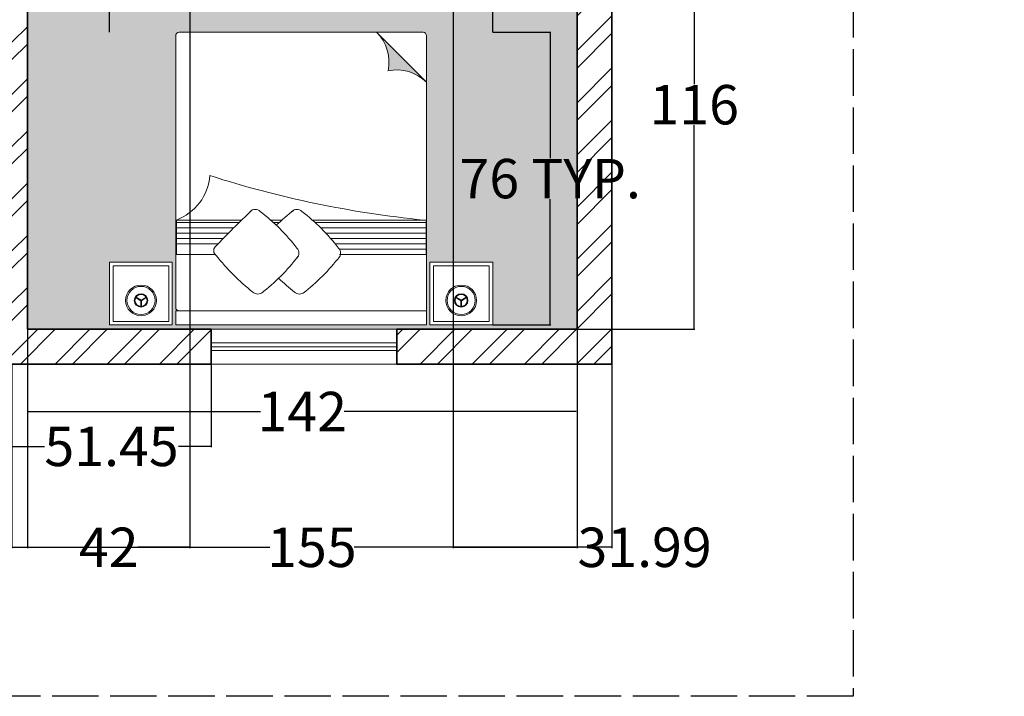
# Model space of a CAD drawing. Units: inches. Extents: x 1410 to 1959, y 5441 to 5968.
# Tile 3 of 5: x 1705 to 1959, y 5441 to 5615. Entities that reach past the tile are written whole.
import ezdxf

# ---------------------------------------------------------------- set-up
doc = ezdxf.new("R2010")
doc.units = ezdxf.units.IN
doc.linetypes.add('ACAD_ISO02W100', pattern=[15, 12, -3])
doc.layers.get('Defpoints').update_dxf_attribs({"linetype": 'ACAD_ISO02W100'})
for name, color, linetype, lineweight in [('00 FURNITURE', 15, 'Continuous', 15), ('A-ANNO-DIMS', 2, 'Continuous', 18), ('A-WALL', 7, 'Continuous', 35), ('A-WALL-PATT', 8, 'Continuous', 13), ('WINDOW', 160, 'Continuous', 13)]:
    doc.layers.add(name, color=color, linetype=linetype, lineweight=lineweight)
doc.layers.add('A-FLOR-PATT', color=9, linetype='Continuous', lineweight=9, true_color=0xafd9aa)
doc.styles.get("Standard").update_dxf_attribs({"font": 'arial.ttf'})
doc.dimstyles.get("Standard").update_dxf_attribs({"dimtxt": 10.18, "dimasz": 0.18, "dimexe": 0.18, "dimexo": 0.0625, "dimgap": 0.09, "dimtad": 0, "dimtih": 1, "dimtoh": 1, "dimdec": 0, "dimzin": 0, "dimdsep": 46, "dimlunit": 3, "dimtxsty": 'Standard', "dimcen": 0.09, "dimadec": 0, "dimazin": 0, "dimtfac": 1, "dimtdec": 0, "dimtofl": 0, "dimtmove": 0, "dimatfit": 3, "dimfxl": 1, "dimtolj": 1, "dimtzin": 0, "dimarcsym": 0})

# ---------------------------------------------------------------- blocks, each defined once
blk = doc.blocks.new('RGWTG')
at = {"layer": '00 FURNITURE'}
for p, q in [((578.23, 3473.51), (577.36, 3475.01)), ((578.36, 3473.58), (577.49, 3475.09)), ((578.23, 3473.58), (577.36, 3472.08)), ((578.36, 3473.51), (577.49, 3472)), ((578.29, 3473.62), (580.03, 3473.62)), ((578.29, 3473.47), (580.03, 3473.47)), ((521.93, 3464.58), (509.03, 3451.68)), ((509.03, 3422.63), (509.03, 3463.68)), ((509.93, 3464.58), (566.4, 3464.58)), ((557.53, 3463.84), (557.53, 3464.49)), ((557.53, 3464.49), (566.4, 3464.49)), ((558.2, 3464.49), (558.2, 3435.82)), ((559.57, 3464.49), (559.57, 3437.25)), ((560.94, 3464.49), (560.94, 3438.58)), ((562.3, 3464.49), (562.3, 3439.83)), ((563.67, 3464.49), (563.67, 3440.99)), ((565.04, 3464.49), (565.04, 3442.08)), ((566.4, 3464.58), (580.98, 3464.58)), ((566.4, 3464.49), (566.4, 3442.08)), ((566.4, 3464.49), (566.4, 3463.84)), ((580.98, 3464.58), (580.98, 3416.72)), ((558.2, 3426.48), (558.2, 3425.04)), ((509.03, 3400.68), (509.03, 3422.63)), ((580.98, 3416.72), (580.98, 3400.68)), ((558.2, 3416.13), (558.2, 3399.95)), ((559.57, 3414.75), (559.57, 3399.95)), ((560.94, 3413.39), (560.94, 3399.95)), ((562.3, 3412.04), (562.3, 3399.95)), ((563.67, 3410.72), (563.67, 3399.95)), ((580.08, 3399.78), (509.93, 3399.78)), ((557.53, 3399.95), (557.53, 3400.6)), ((566.4, 3399.95), (557.53, 3399.95)), ((566.4, 3400.6), (566.4, 3399.95)), ((578.23, 3390.78), (577.36, 3392.29)), ((578.36, 3390.86), (577.49, 3392.36)), ((578.23, 3390.86), (577.36, 3389.36)), ((578.36, 3390.78), (577.49, 3389.28)), ((578.29, 3390.9), (580.03, 3390.9)), ((578.29, 3390.74), (580.03, 3390.74))]:
    blk.add_line(p, q, dxfattribs=at)
for points in [[(568.43, 3465.48), (584.63, 3465.48), (584.63, 3481.68), (568.43, 3481.68)], [(569.33, 3466.38), (583.73, 3466.38), (583.73, 3480.78), (569.33, 3480.78)], [(580.98, 3399.78), (584.63, 3399.78), (584.63, 3464.58), (580.98, 3464.58)], [(568.43, 3398.88), (584.63, 3398.88), (584.63, 3382.68), (568.43, 3382.68)], [(569.33, 3397.98), (583.73, 3397.98), (583.73, 3383.58), (569.33, 3383.58)]]:
    blk.add_lwpolyline(points, close=True, dxfattribs=at)
for points in [[(566.52, 3464.49), (557.53, 3464.49), (557.53, 3435.08)], [(557.53, 3427.21), (557.53, 3424.3)], [(557.53, 3416.82), (557.53, 3399.95), (566.4, 3399.95), (566.4, 3409.94)]]:
    blk.add_lwpolyline(points, dxfattribs=at)
for centre, radius in [((578.29, 3473.54), 3.97), ((578.29, 3473.54), 3.63), ((578.29, 3473.54), 1.74), ((578.29, 3473.54), 1.56), ((578.29, 3390.82), 3.97), ((578.29, 3390.82), 3.63), ((578.29, 3390.82), 1.74), ((578.29, 3390.82), 1.56)]:
    blk.add_circle(centre, radius, dxfattribs=at)
for centre, radius, start, end in [((509.93, 3463.68), 0.9, 90, 180), ((529.65, 3456.88), 10.9, 135.0361, 191.9278), ((290.56, 3490.52), 268.3, 342.2214, 354.2925), ((516.73, 3443.97), 10.9, 78.0722, 134.9639), ((566.05, 3440.57), 1.82, 45, 135), ((533.58, 3399.31), 54.32, 37.931, 52.069), ((598.15, 3399.01), 54.32, 127.931, 142.069), ((556.59, 3431.11), 1.82, 135, 225), ((574.84, 3431.77), 1.82, 315, 45), ((597.87, 3463.6), 54.32, 217.931, 224.141), ((598.15, 3388.23), 54.32, 127.931, 142.069), ((566.05, 3429.78), 1.82, 45, 135), ((533.58, 3388.53), 54.32, 37.931, 52.069), ((533.28, 3463.88), 54.32, 316.32, 322.069), ((556.59, 3420.33), 1.82, 135, 225), ((574.84, 3420.99), 1.82, 315, 45), ((765.33, 3619.75), 290.45, 223.6069, 226.2326), ((533.28, 3453.1), 54.32, 307.931, 322.069), ((565.44, 3411.05), 1.47, 225.9674, 326.8337), ((545.02, 3395.29), 13.35, 20.4224, 85.5825), ((509.93, 3400.68), 0.9, 180, 270), ((580.08, 3400.68), 0.9, 270, 0)]:
    blk.add_arc(centre, radius, start, end, dxfattribs=at)
blk = doc.blocks.new('WIN-48IN')
for p, q in [((48, 9), (0, 9)), ((0, 5.5), (48, 5.5)), ((0, 4.5), (48, 4.5)), ((0, 3.5), (48, 3.5)), ((0, 0), (48, 0))]:
    blk.add_line(p, q)
blk = doc.blocks.new('*D14')
at = {"layer": 'A-ANNO-DIMS', "color": 0, "lineweight": -2, "transparency": 16777216}
for p, q in [((1728.31, 5612.14), (1728.31, 5627.11)), ((1728.49, 5626.93), (1827.13, 5626.93)), ((1827.31, 5612.14), (1827.31, 5627.11)), ((1827.31, 5626.93), (1827.49, 5626.93))]:
    blk.add_line(p, q, dxfattribs=at)
at = {"layer": 'A-ANNO-DIMS', "color": 0, "transparency": 16777216}
for points in [[(1728.49, 5626.96), (1728.49, 5626.9), (1728.31, 5626.93)], [(1827.13, 5626.96), (1827.13, 5626.9), (1827.31, 5626.93)]]:
    blk.add_solid(points, dxfattribs=at)
at = {"layer": 'Defpoints', "color": 0, "transparency": 16777216}
for p in [(1827.31, 5626.93), (1728.31, 5612.08), (1827.31, 5612.08)]:
    blk.add_point(p, dxfattribs=at)
at = {"layer": 'A-ANNO-DIMS', "color": 0, "transparency": 16777216, "insert": (1896.77, 5626.93), "char_height": 10.18, "attachment_point": 5}
blk.add_mtext('\\A1;BED GROUP 99 TYP.', dxfattribs=at)
blk = doc.blocks.new('*D15')
at = {"layer": 'A-ANNO-DIMS', "color": 0, "lineweight": -2, "transparency": 16777216}
for p, q in [((1827.37, 5612.08), (1842.34, 5612.08)), ((1842.16, 5611.9), (1842.16, 5579.57)), ((1842.16, 5536.66), (1842.16, 5568.99)), ((1827.37, 5536.48), (1842.34, 5536.48))]:
    blk.add_line(p, q, dxfattribs=at)
at = {"layer": 'A-ANNO-DIMS', "color": 0, "transparency": 16777216}
for points in [[(1842.13, 5611.9), (1842.19, 5611.9), (1842.16, 5612.08)], [(1842.13, 5536.66), (1842.19, 5536.66), (1842.16, 5536.48)]]:
    blk.add_solid(points, dxfattribs=at)
at = {"layer": 'Defpoints', "color": 0, "transparency": 16777216}
for p in [(1827.31, 5612.08), (1827.31, 5536.48), (1842.16, 5536.48)]:
    blk.add_point(p, dxfattribs=at)
at = {"layer": 'A-ANNO-DIMS', "color": 0, "transparency": 16777216, "insert": (1842.16, 5574.28), "char_height": 10.18, "attachment_point": 5}
blk.add_mtext('\\A1;76 TYP.', dxfattribs=at)
blk = doc.blocks.new('*D26')
at = {"layer": 'A-ANNO-DIMS', "color": 0, "lineweight": -2, "transparency": 16777216}
for p, q in [((1703.09, 5526.3), (1703.09, 5478.87)), ((1858.09, 5526.3), (1858.09, 5478.87)), ((1703.27, 5479.05), (1769.7, 5479.05)), ((1857.91, 5479.05), (1791.49, 5479.05))]:
    blk.add_line(p, q, dxfattribs=at)
at = {"layer": 'A-ANNO-DIMS', "color": 0, "transparency": 16777216}
for points in [[(1703.27, 5479.08), (1703.27, 5479.02), (1703.09, 5479.05)], [(1857.91, 5479.08), (1857.91, 5479.02), (1858.09, 5479.05)]]:
    blk.add_solid(points, dxfattribs=at)
at = {"layer": 'Defpoints', "color": 0, "transparency": 16777216}
for p in [(1703.09, 5526.37), (1858.09, 5526.37), (1858.09, 5479.05)]:
    blk.add_point(p, dxfattribs=at)
at = {"layer": 'A-ANNO-DIMS', "color": 0, "transparency": 16777216, "insert": (1780.59, 5479.05), "char_height": 10.18, "attachment_point": 5}
blk.add_mtext('\\A1;155', dxfattribs=at)
blk = doc.blocks.new('*D28')
at = {"layer": 'A-ANNO-DIMS', "color": 0, "lineweight": -2, "transparency": 16777216}
for p, q in [((1817.1, 5913.3), (1817.1, 5478.87)), ((1849.09, 5913.3), (1849.09, 5478.87)), ((1817.28, 5479.05), (1848.91, 5479.05)), ((1849.09, 5479.05), (1849.27, 5479.05))]:
    blk.add_line(p, q, dxfattribs=at)
at = {"layer": 'A-ANNO-DIMS', "color": 0, "transparency": 16777216}
for points in [[(1817.28, 5479.08), (1817.28, 5479.02), (1817.1, 5479.05)], [(1848.91, 5479.08), (1848.91, 5479.02), (1849.09, 5479.05)]]:
    blk.add_solid(points, dxfattribs=at)
at = {"layer": 'Defpoints', "color": 0, "transparency": 16777216}
for p in [(1817.1, 5913.37), (1849.09, 5913.37), (1849.09, 5479.05)]:
    blk.add_point(p, dxfattribs=at)
at = {"layer": 'A-ANNO-DIMS', "color": 0, "transparency": 16777216, "insert": (1866.55, 5479.05), "char_height": 10.18, "attachment_point": 5}
blk.add_mtext('\\A1;31.99', dxfattribs=at)
blk = doc.blocks.new('*D31')
at = {"layer": 'A-ANNO-DIMS', "color": 0, "lineweight": -2, "transparency": 16777216}
for p, q in [((1703.09, 5526.3), (1703.09, 5504.94)), ((1754.54, 5526.3), (1754.54, 5504.94)), ((1703.27, 5505.12), (1711.51, 5505.12)), ((1754.36, 5505.12), (1746.12, 5505.12))]:
    blk.add_line(p, q, dxfattribs=at)
at = {"layer": 'A-ANNO-DIMS', "color": 0, "transparency": 16777216}
for points in [[(1703.27, 5505.15), (1703.27, 5505.09), (1703.09, 5505.12)], [(1754.36, 5505.15), (1754.36, 5505.09), (1754.54, 5505.12)]]:
    blk.add_solid(points, dxfattribs=at)
at = {"layer": 'Defpoints', "color": 0, "transparency": 16777216}
for p in [(1703.09, 5526.37), (1754.54, 5526.37), (1703.09, 5505.12)]:
    blk.add_point(p, dxfattribs=at)
at = {"layer": 'A-ANNO-DIMS', "color": 0, "transparency": 16777216, "insert": (1728.82, 5505.12), "char_height": 10.18, "attachment_point": 5}
blk.add_mtext('\\A1;51.45', dxfattribs=at)
blk = doc.blocks.new('*D41')
at = {"layer": 'A-ANNO-DIMS', "color": 0, "lineweight": -2, "transparency": 16777216}
for p, q in [((1849.16, 5651.37), (1879.55, 5651.37)), ((1879.37, 5651.19), (1879.37, 5598.65)), ((1879.37, 5535.55), (1879.37, 5588.08)), ((1849.16, 5535.37), (1879.55, 5535.37))]:
    blk.add_line(p, q, dxfattribs=at)
at = {"layer": 'A-ANNO-DIMS', "color": 0, "transparency": 16777216}
for points in [[(1879.34, 5651.19), (1879.4, 5651.19), (1879.37, 5651.37)], [(1879.34, 5535.55), (1879.4, 5535.55), (1879.37, 5535.37)]]:
    blk.add_solid(points, dxfattribs=at)
at = {"layer": 'Defpoints', "color": 0, "transparency": 16777216}
for p in [(1849.09, 5651.37), (1879.37, 5651.37), (1849.09, 5535.37)]:
    blk.add_point(p, dxfattribs=at)
at = {"layer": 'A-ANNO-DIMS', "color": 0, "transparency": 16777216, "insert": (1879.37, 5593.37), "char_height": 10.18, "attachment_point": 5}
blk.add_mtext('\\A1;116', dxfattribs=at)
blk = doc.blocks.new('*D42')
at = {"layer": 'A-ANNO-DIMS', "color": 0, "lineweight": -2, "transparency": 16777216}
for p, q in [((1707.09, 5535.3), (1707.09, 5513.94)), ((1849.09, 5535.3), (1849.09, 5513.94)), ((1707.27, 5514.12), (1767.29, 5514.12)), ((1848.91, 5514.12), (1788.9, 5514.12))]:
    blk.add_line(p, q, dxfattribs=at)
at = {"layer": 'A-ANNO-DIMS', "color": 0, "transparency": 16777216}
for points in [[(1707.27, 5514.15), (1707.27, 5514.09), (1707.09, 5514.12)], [(1848.91, 5514.15), (1848.91, 5514.09), (1849.09, 5514.12)]]:
    blk.add_solid(points, dxfattribs=at)
at = {"layer": 'Defpoints', "color": 0, "transparency": 16777216}
for p in [(1707.09, 5535.37), (1849.09, 5535.37), (1707.09, 5514.12)]:
    blk.add_point(p, dxfattribs=at)
at = {"layer": 'A-ANNO-DIMS', "color": 0, "transparency": 16777216, "insert": (1778.09, 5514.12), "char_height": 10.18, "attachment_point": 5}
blk.add_mtext('\\A1;142', dxfattribs=at)
blk = doc.blocks.new('*D46')
at = {"layer": 'A-ANNO-DIMS', "color": 0, "lineweight": -2, "transparency": 16777216}
for p, q in [((1707.09, 5711.3), (1707.09, 5478.87)), ((1749.09, 5699.3), (1749.09, 5478.87)), ((1707.27, 5479.05), (1720.56, 5479.05)), ((1748.91, 5479.05), (1735.63, 5479.05))]:
    blk.add_line(p, q, dxfattribs=at)
at = {"layer": 'A-ANNO-DIMS', "color": 0, "transparency": 16777216}
for points in [[(1707.27, 5479.08), (1707.27, 5479.02), (1707.09, 5479.05)], [(1748.91, 5479.08), (1748.91, 5479.02), (1749.09, 5479.05)]]:
    blk.add_solid(points, dxfattribs=at)
at = {"layer": 'Defpoints', "color": 0, "transparency": 16777216}
for p in [(1707.09, 5711.37), (1749.09, 5699.37), (1749.09, 5479.05)]:
    blk.add_point(p, dxfattribs=at)
at = {"layer": 'A-ANNO-DIMS', "color": 0, "transparency": 16777216, "insert": (1728.09, 5479.05), "char_height": 10.18, "attachment_point": 5}
blk.add_mtext('\\A1;42', dxfattribs=at)

msp = doc.modelspace()

# ---------------------------------------------------------------- hatches: boundary and pattern name
at = {"layer": 'A-FLOR-PATT', "transparency": 33554534}
h = msp.add_hatch(color=256, dxfattribs=at)
h.dxf.hatch_style = 1
h.paths.add_polyline_path([(1849.0942, 5913.3659), (1817.1029, 5913.3659), (1769.1029, 5913.3659), (1769.1029, 5913.3659), (1707.0942, 5913.3659), (1707.0942, 5787.3659), (1703.0942, 5787.3659), (1703.0942, 5799.3659), (1631.0942, 5799.3659), (1631.0942, 5787.3659), (1627.0942, 5787.3659), (1627.0942, 5889.3659), (1519.0989, 5889.3659), (1519.0989, 5816.4745), (1495.0981, 5816.4745), (1495.0981, 5809.856), (1495.0942, 5751.3659), (1631.0942, 5751.3659), (1631.0942, 5747.3659), (1495.0942, 5747.3659), (1495.0942, 5702.5811), (1495.0984, 5654.5768), (1495.0942, 5603.3659), (1667.0942, 5603.3659), (1667.0942, 5594.3659), (1650.778, 5594.3659), (1650.778, 5558.3659), (1703.0942, 5558.3659), (1703.0942, 5594.3659), (1703.0942, 5711.3659), (1707.0942, 5711.3659), (1707.0942, 5535.3659), (1754.5413, 5535.3659), (1802.541, 5535.3658), (1802.5413, 5535.3658), (1802.5413, 5535.3659), (1849.0942, 5535.3659), (1849.0942, 5651.3659), (1743.0942, 5651.3659), (1743.0942, 5655.3659), (1849.0942, 5655.3659), (1849.0942, 5665.4579), (1849.0942, 5689.4579), (1849.0942, 5699.3659), (1801.0942, 5699.3659), (1801.0942, 5685.3659), (1797.0942, 5685.3659), (1797.0942, 5699.3659), (1783.0942, 5699.3659), (1783.0942, 5703.3659), (1849.0942, 5703.3659), (1849.0942, 5716.9764), (1849.123, 5716.9764), (1849.123, 5740.9654), (1849.0942, 5740.9654), (1849.0942, 5747.3659), (1753.0942, 5747.3659), (1753.0942, 5699.3659), (1749.0942, 5699.3659), (1749.0942, 5747.3659), (1707.0942, 5747.3659), (1691.0942, 5747.3659), (1691.0942, 5751.3659), (1707.0942, 5751.3659), (1849.0942, 5751.3659)])
h.paths.add_polyline_path([(1533.4842, 5711.1518), (1533.4842, 5637.9201), (1534.7464, 5637.9201), (1534.7464, 5640.1099, -0.41421356), (1536.9363, 5642.2998), (1558.8347, 5642.2998, -0.41421356), (1561.0246, 5640.1099), (1561.0246, 5637.9201), (1563.2144, 5637.9201, -0.41421356), (1565.4042, 5635.7302), (1565.4042, 5609.4519, -0.41421356), (1563.2144, 5607.2621), (1532.5566, 5607.2621, -0.41421356), (1530.3668, 5609.4519), (1530.3668, 5635.4862), (1529.1045, 5635.4862), (1529.1045, 5633.2964, -0.41421356), (1526.9147, 5631.1065), (1500.6363, 5631.1065, -0.41421356), (1498.4465, 5633.2964), (1498.4465, 5715.5315, -0.41421356), (1500.6363, 5717.7213), (1526.9147, 5717.7213, -0.41421356), (1529.1045, 5715.5315), (1529.1045, 5713.3417), (1531.2944, 5713.3417, -0.41421356)], flags=16)
h.paths.add_polyline_path([(1771.0631, 5793.9619), (1771.0631, 5835.0118), (1771.0631, 5856.9619, -0.41421356), (1771.9631, 5857.8619), (1842.1181, 5857.8619, -0.41421356), (1843.0181, 5856.9619), (1843.0181, 5857.8619), (1846.6631, 5857.8619), (1846.6631, 5793.0619), (1843.0181, 5793.0619), (1828.4381, 5793.0619), (1771.9631, 5793.0619, -0.41421356)], flags=16)
h.paths.add_polyline_path([(1771.0631, 5805.9671, 0.25346465), (1781.0166, 5803.0153, 0.25379956), (1783.9781, 5793.0522)], flags=16)
h.paths.add_polyline_path([(1746.3058, 5612.0795), (1768.2559, 5612.0795), (1809.3058, 5612.0795, -0.41421356), (1810.2058, 5611.1795), (1810.2058, 5554.7045), (1810.2058, 5540.1245), (1810.2058, 5536.4795), (1745.4058, 5536.4795), (1745.4058, 5540.1245), (1746.3058, 5540.1245, -0.41421356), (1745.4058, 5541.0245), (1745.4058, 5611.1795, -0.41421356)], flags=16)
h.paths.add_polyline_path([(1819.5646, 5793.1537), (1819.5646, 5793.8054, 0.05271893), (1808.0815, 5849.0458, 0.29223153), (1819.5646, 5857.6981), (1828.4381, 5857.6981), (1828.4381, 5857.0464), (1828.4381, 5847.601, -0.06332793), (1838.1593, 5837.9401, -0.38046479), (1838.3062, 5835.5217, -0.02593615), (1834.5989, 5831.2824, -0.02509022), (1838.1593, 5827.1584, -0.38046478), (1838.3062, 5824.74, -0.05941785), (1829.2061, 5815.646, -0.11763956), (1828.4381, 5815.2914), (1828.4381, 5793.1537)], flags=0)
h.paths.add_polyline_path([(1819.5646, 5793.1537), (1819.5646, 5822.5662, -0.01603557), (1817.3363, 5825.2436, -0.4295765), (1817.4052, 5827.8865, -0.01537126), (1819.5646, 5830.4335), (1819.5646, 5833.3479, -0.01603557), (1817.3363, 5836.0254, -0.48413611), (1817.6682, 5838.8652, 0.00079305), (1817.0318, 5838.199, 0.26524804), (1817.0526, 5836.3926, 0.02736634), (1820.9176, 5831.8795, 0.02734261), (1817.0221, 5827.3996, 0.26229506), (1817.0526, 5825.6108, 0.06555279), (1827.0712, 5815.5721), (1827.0712, 5793.1537)], flags=0)
h.paths.add_polyline_path([(1830.4631, 5775.9619), (1830.4631, 5792.1619), (1846.6631, 5792.1619), (1846.6631, 5775.9619)], flags=16)
h.paths.add_polyline_path([(1831.3631, 5776.8619), (1831.3631, 5791.2619), (1845.7631, 5791.2619), (1845.7631, 5776.8619)], flags=0)
h.paths.add_polyline_path([(1836.6983, 5784.1006, -1), (1843.9547, 5784.1006, -1)], flags=0)
h.paths.add_polyline_path([(1819.2615, 5682.5311, -0.25820517), (1830.2865, 5687.0962, -0.1716359), (1835.799, 5683.9093), (1838.1615, 5683.9093), (1838.1615, 5688.0436, -0.41421356), (1839.1458, 5689.028), (1845.4458, 5689.028, -0.41421356), (1846.4302, 5688.0436), (1846.4302, 5671.8999, -0.41421356), (1845.4458, 5670.9155), (1839.1458, 5670.9155, -0.41421356), (1838.1615, 5671.8999), (1838.1615, 5676.0343), (1835.799, 5676.0343, -0.1716359), (1830.2865, 5672.8474, -0.25820517), (1819.2615, 5677.4124)], flags=16)
h.paths.add_polyline_path([(1820.8043, 5682.5681, -0.21038447), (1830.2865, 5685.5212, -0.1716359), (1835.799, 5682.3343), (1835.799, 5677.6093, -0.1716359), (1830.2865, 5674.4224, -0.21038447), (1820.8043, 5677.3755)], flags=0)
h.paths.add_polyline_path([(1842.0614, 5784.0231), (1841.8811, 5784.0231, -0.54460611), (1839.6163, 5782.7155), (1839.5262, 5782.5594, 0.54796211)], flags=0)
h.paths.add_polyline_path([(1840.3713, 5784.1781), (1840.3265, 5784.2556), (1840.2818, 5784.1781)], flags=0)
h.paths.add_polyline_path([(1830.4631, 5858.7619), (1830.4631, 5874.9619), (1846.6631, 5874.9619), (1846.6631, 5858.7619)], flags=16)
h.paths.add_polyline_path([(1831.3631, 5859.6619), (1831.3631, 5874.0619), (1845.7631, 5874.0619), (1845.7631, 5859.6619)], flags=0)
h.paths.add_polyline_path([(1755.6206, 5556.6903, -0.00089292), (1756.3396, 5557.4382), (1745.5695, 5557.4382), (1745.5695, 5554.7045), (1746.2212, 5554.7045), (1755.5673, 5554.7045, -0.38881883)], flags=0)
h.paths.add_polyline_path([(1810.114, 5563.578), (1810.114, 5554.7045), (1809.4622, 5554.7045), (1787.9762, 5554.7045, -0.11778508), (1787.6251, 5553.9338, -0.05941785), (1778.5249, 5544.8398, -0.37985907), (1776.1092, 5544.9833, -0.02509022), (1771.9852, 5548.5437, 0.03343123), (1776.8399, 5553.9365, 0.30845915), (1776.98, 5555.985, 0.04782679), (1769.9197, 5563.578), (1772.8341, 5563.578, -0.01537126), (1775.3811, 5565.7373, -0.4295765), (1778.024, 5565.8063, -0.01603557), (1780.7015, 5563.578)], flags=0)
h.paths.add_polyline_path([(1728.3058, 5552.6795), (1744.5058, 5552.6795), (1744.5058, 5536.4795), (1728.3058, 5536.4795)], flags=16)
h.paths.add_polyline_path([(1810.2058, 5599.1742, 0.25346465), (1800.2523, 5602.126, 0.25379956), (1797.2908, 5612.0892)], flags=16)
h.paths.add_polyline_path([(1843.9547, 5866.8231, -1), (1836.6983, 5866.8231, -1)], flags=0)
h.paths.add_polyline_path([(1729.2058, 5551.7795), (1743.6058, 5551.7795), (1743.6058, 5537.3795), (1729.2058, 5537.3795)], flags=0)
h.paths.add_polyline_path([(1839.4821, 5865.5155), (1840.237, 5866.8231), (1839.4821, 5868.1307, 0.25464572), (1838.77, 5866.8231, 0.25464572)], flags=0)
h.paths.add_polyline_path([(1842.0614, 5866.7456), (1840.3713, 5866.7456), (1839.5262, 5865.2819, 0.54796211)], flags=0)
h.paths.add_polyline_path([(1732.8163, 5542.8161, -1), (1740.0727, 5542.8161, -1)], flags=0)
h.paths.add_polyline_path([(1737.8296, 5543.5262), (1736.522, 5542.7713), (1736.522, 5541.2615, 0.39969799), (1738.001, 5542.8161, 0.11900365)], flags=0)
h.paths.add_polyline_path([(1738.1811, 5542.8161, -1), (1734.7079, 5542.8161, -1)], flags=0)
h.paths.add_polyline_path([(1736.4445, 5542.9056), (1736.367, 5542.9503), (1736.367, 5542.8608)], flags=0)
h.paths.add_polyline_path([(1811.1058, 5552.6795), (1827.3058, 5552.6795), (1827.3058, 5536.4795), (1811.1058, 5536.4795)], flags=16)
h.paths.add_polyline_path([(1812.0058, 5551.7795), (1826.4058, 5551.7795), (1826.4058, 5537.3795), (1812.0058, 5537.3795)], flags=0)
h.paths.add_polyline_path([(1815.5388, 5542.8161, -1), (1822.7952, 5542.8161, -1)], flags=0)
h.paths.add_polyline_path([(1820.5521, 5543.5262), (1819.2445, 5542.7713), (1819.2445, 5541.2615, 0.39969799), (1820.7235, 5542.8161, 0.11900365)], flags=0)
h.paths.add_polyline_path([(1820.9036, 5542.8161, -1), (1817.4304, 5542.8161, -1)], flags=0)
h.paths.add_polyline_path([(1819.167, 5542.9056), (1819.0895, 5542.9503), (1819.0895, 5542.8608)], flags=0)
h.paths.add_polyline_path([(1707.0264, 5710.8395), (1750.0905, 5710.8395), (1750.0905, 5723.2037), (1707.0264, 5723.2037)], flags=25)
h.paths.add_polyline_path([(1786.4108, 5658.162), (1818.7518, 5658.162), (1818.7518, 5680.5262), (1786.4108, 5680.5262)], flags=24)
h.paths.add_polyline_path([(1787.0609, 5715.7465), (1838.4906, 5715.7465), (1838.4906, 5738.1353), (1787.0609, 5738.1353)], flags=24)
h.paths.add_polyline_path([(1743.8116, 5616.0244), (1813.7243, 5616.0244), (1813.7243, 5649.6076), (1743.8116, 5649.6076)], flags=24)
h.paths.add_polyline_path([(1719.2569, 5867.7974), (1789.1696, 5867.7974), (1789.1696, 5901.3806), (1719.2569, 5901.3806)], flags=24)
h.paths.add_polyline_path([(1562.3198, 5677.907), (1619.4324, 5677.907), (1619.4324, 5711.4902), (1562.3198, 5711.4902)], flags=24)
h.paths.add_polyline_path([(1544.1706, 5816.5955), (1604.3036, 5816.5955), (1604.3036, 5850.1787), (1544.1706, 5850.1787)], flags=24)
at = {"layer": 'A-WALL-PATT'}
h = msp.add_hatch(dxfattribs=at)
h.set_pattern_fill('ANSI32', color=256)
h.paths.add_polyline_path([(1526.9987, 5922.3659), (1486.0942, 5922.3659), (1486.0942, 5857.8561), (1495.0942, 5857.8561), (1495.0942, 5913.3659), (1526.9987, 5913.3659)])
h.paths.add_polyline_path([(1769.1029, 5922.3659), (1574.9987, 5922.3659), (1574.9987, 5913.3659), (1574.9993, 5913.3659), (1627.0942, 5913.3659), (1627.0942, 5787.3659), (1631.0942, 5787.3659), (1631.0942, 5913.3659), (1703.0942, 5913.3659), (1703.0942, 5787.3659), (1707.0942, 5787.3659), (1707.0942, 5913.3659), (1769.1029, 5913.3659)])
h.paths.add_polyline_path([(1858.0942, 5922.3659), (1817.1029, 5922.3659), (1817.1029, 5913.3659), (1849.0942, 5913.3659), (1849.0942, 5751.3659), (1707.0942, 5751.3659), (1691.0942, 5751.3659), (1691.0942, 5747.3659), (1707.0942, 5747.3659), (1849.0942, 5747.3659), (1849.0942, 5740.9764), (1858.0942, 5740.9764)])
h.paths.add_polyline_path([(1495.0942, 5809.8561), (1486.0981, 5809.8561), (1486.0981, 5809.856), (1486.0942, 5702.5811), (1495.0942, 5702.5811), (1495.0942, 5747.3659), (1631.0942, 5747.3659), (1631.0942, 5751.3659), (1495.0942, 5751.3659)])
h.paths.add_polyline_path([(1495.0942, 5654.5811), (1486.0984, 5654.5811), (1486.0984, 5654.5768), (1486.0942, 5594.3659), (1667.0942, 5594.3659), (1667.0942, 5603.3659), (1495.0942, 5603.3659)])
h.paths.add_polyline_path([(1858.0942, 5665.4579), (1849.0942, 5665.4579), (1849.0942, 5655.3659), (1743.0942, 5655.3659), (1743.0942, 5651.3659), (1849.0942, 5651.3659), (1849.0942, 5535.3659), (1802.5413, 5535.3659), (1802.5413, 5526.3659), (1858.0942, 5526.3659)])
h.paths.add_polyline_path([(1858.0942, 5716.9654), (1849.0942, 5716.9654), (1849.0942, 5703.3659), (1783.0942, 5703.3659), (1783.0942, 5699.3659), (1797.0942, 5699.3659), (1797.0942, 5685.3659), (1801.0942, 5685.3659), (1801.0942, 5699.3659), (1849.0942, 5699.3659), (1849.0942, 5689.4579), (1858.0942, 5689.4579)])
h.paths.add_polyline_path([(1753.0942, 5747.3659), (1749.0942, 5747.3659), (1749.0942, 5699.3659), (1753.0942, 5699.3659)])
h.paths.add_polyline_path([(1707.0942, 5711.3659), (1703.0942, 5711.3659), (1703.0942, 5594.3659), (1703.0942, 5526.3659), (1754.5413, 5526.3659), (1754.5413, 5535.3658), (1754.541, 5535.3658), (1707.0942, 5535.3659)])

# ---------------------------------------------------------------- linework, layer by layer
at = {"layer": 'A-WALL'}
for p, q in [((1707.0942, 5711.3659), (1707.0942, 5535.3659)), ((1858.0942, 5665.4579), (1858.0942, 5526.3659)), ((1849.0942, 5651.3659), (1849.0942, 5535.3659)), ((1754.5413, 5535.3659), (1707.0942, 5535.3659)), ((1754.5413, 5535.3659), (1754.5413, 5526.3659)), ((1849.0942, 5535.3659), (1802.5413, 5535.3659)), ((1802.5413, 5535.3659), (1802.5413, 5526.3659)), ((1754.5413, 5526.3659), (1703.0942, 5526.3659)), ((1858.0942, 5526.3659), (1802.5413, 5526.3659))]:
    msp.add_line(p, q, dxfattribs=at)
at = {"layer": 'Defpoints'}
msp.add_lwpolyline([(1409.7428, 5967.6887), (1920.4745, 5967.6887), (1920.4745, 5440.571), (1409.7428, 5440.571)], close=True, dxfattribs=at)

# ---------------------------------------------------------------- block references
at = {"layer": '00 FURNITURE', "rotation": 270}
msp.add_blockref('RGWTG', (-1654.3769, 6121.1089), dxfattribs=at)
at = {"layer": 'WINDOW', "rotation": 180}
msp.add_blockref('WIN-48IN', (1802.541, 5535.3658), dxfattribs=at)

# ---------------------------------------------------------------- dimensions: what is measured, and where the dimension line sits
at = {"layer": 'A-ANNO-DIMS'}
for base, p1, p2, override, picture, middle in [((1849.0942, 5479.0498), (1817.1029, 5913.3659), (1849.0942, 5913.3659), {"dimdec": 2, "dimlfac": 1, "dimrnd": 0, "dimzin": 0, "dimdsep": 46, "dimlunit": 2}, '*D28', (1866.5473, 5479.0498)), ((1749.0942, 5479.0498), (1707.0942, 5711.3659), (1749.0942, 5699.3659), {"dimdec": 0, "dimlfac": 1, "dimrnd": 0, "dimzin": 0, "dimdsep": 46, "dimlunit": 2}, '*D46', (1728.0942, 5479.0498)), ((1858.0942, 5479.0498), (1703.0942, 5526.3659), (1858.0942, 5526.3659), {"dimdec": 0, "dimlfac": 1, "dimrnd": 0, "dimzin": 0, "dimdsep": 46, "dimlunit": 2}, '*D26', (1780.5942, 5479.0498))]:
    dim = msp.add_linear_dim(base=base, p1=p1, p2=p2, dimstyle='Standard', override=override, dxfattribs=at)
    dim.commit()
    dim.dimension.update_dxf_attribs({"geometry": picture, "text_midpoint": middle})
dim = msp.add_linear_dim(base=(1827.3058, 5626.9295), p1=(1728.3058, 5612.0795), p2=(1827.3058, 5612.0795), text='BED GROUP <> TYP.', dimstyle='Standard', override={"dimdec": 0, "dimlfac": 1, "dimrnd": 0, "dimzin": 0, "dimdsep": 46, "dimlunit": 2}, dxfattribs=at)
dim.commit()
dim.dimension.update_dxf_attribs({"geometry": '*D14', "text_midpoint": (1896.7734, 5626.9295)})
for base, p1, p2, angle, override, picture, middle in [((1879.373, 5651.3659), (1849.0942, 5535.3659), (1849.0942, 5651.3659), 90, {"dimdec": 0, "dimlfac": 1, "dimrnd": 0, "dimzin": 0, "dimdsep": 46, "dimlunit": 2}, '*D41', (1879.373, 5593.3659)), ((1707.0942, 5514.1159), (1849.0942, 5535.3659), (1707.0942, 5535.3659), 180, {"dimdec": 0, "dimlfac": 1, "dimrnd": 0, "dimzin": 0, "dimdsep": 46, "dimlunit": 2}, '*D42', (1778.0942, 5514.1159)), ((1703.0942, 5505.1159), (1754.5413, 5526.3659), (1703.0942, 5526.3659), 180, {"dimdec": 2, "dimlfac": 1, "dimrnd": 0, "dimzin": 0, "dimdsep": 46, "dimlunit": 2}, '*D31', (1728.8178, 5505.1159))]:
    dim = msp.add_linear_dim(base=base, p1=p1, p2=p2, angle=angle, dimstyle='Standard', override=override, dxfattribs=at)
    dim.commit()
    dim.dimension.update_dxf_attribs({"geometry": picture, "text_midpoint": middle})
dim = msp.add_linear_dim(base=(1842.1558, 5536.4795), p1=(1827.3058, 5612.0795), p2=(1827.3058, 5536.4795), angle=270, text='<> TYP.', dimstyle='Standard', override={"dimdec": 0, "dimlfac": 1, "dimrnd": 0, "dimzin": 0, "dimdsep": 46, "dimlunit": 2}, dxfattribs=at)
dim.commit()
dim.dimension.update_dxf_attribs({"geometry": '*D15', "text_midpoint": (1842.1558, 5574.2795)})

doc.saveas('drawing.dxf')
